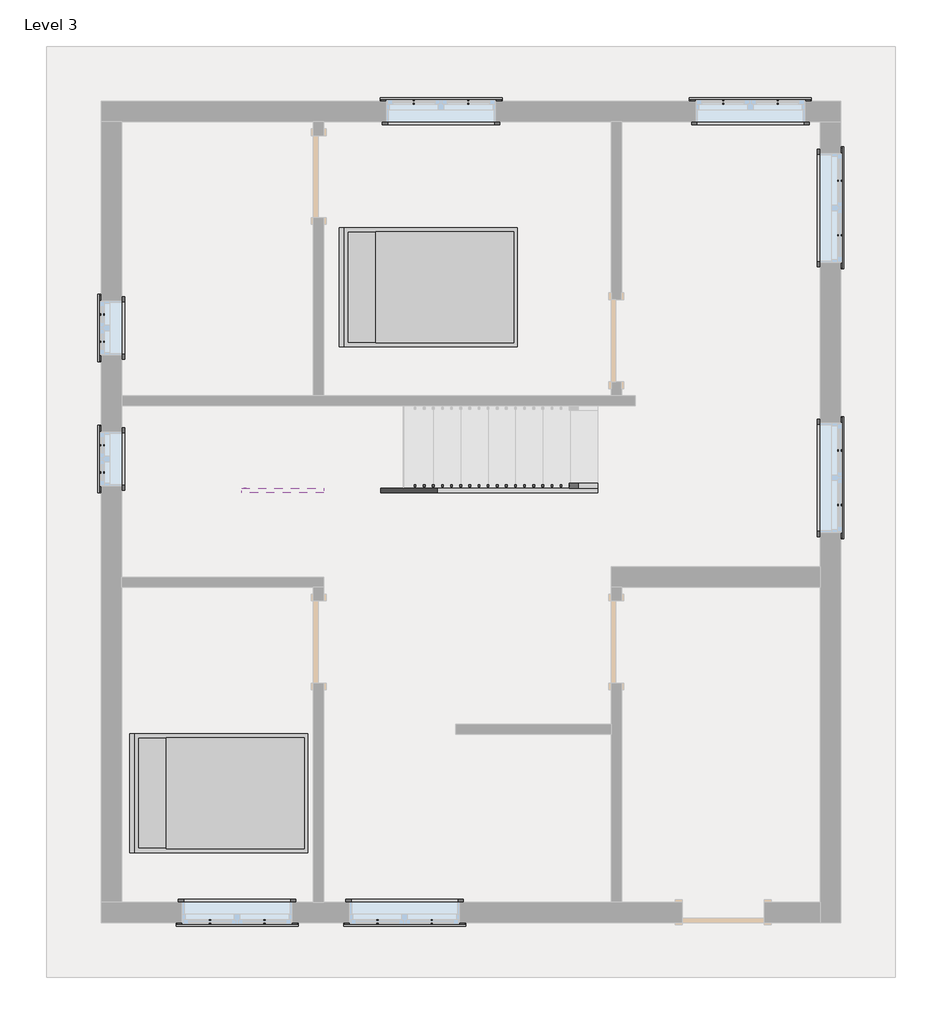
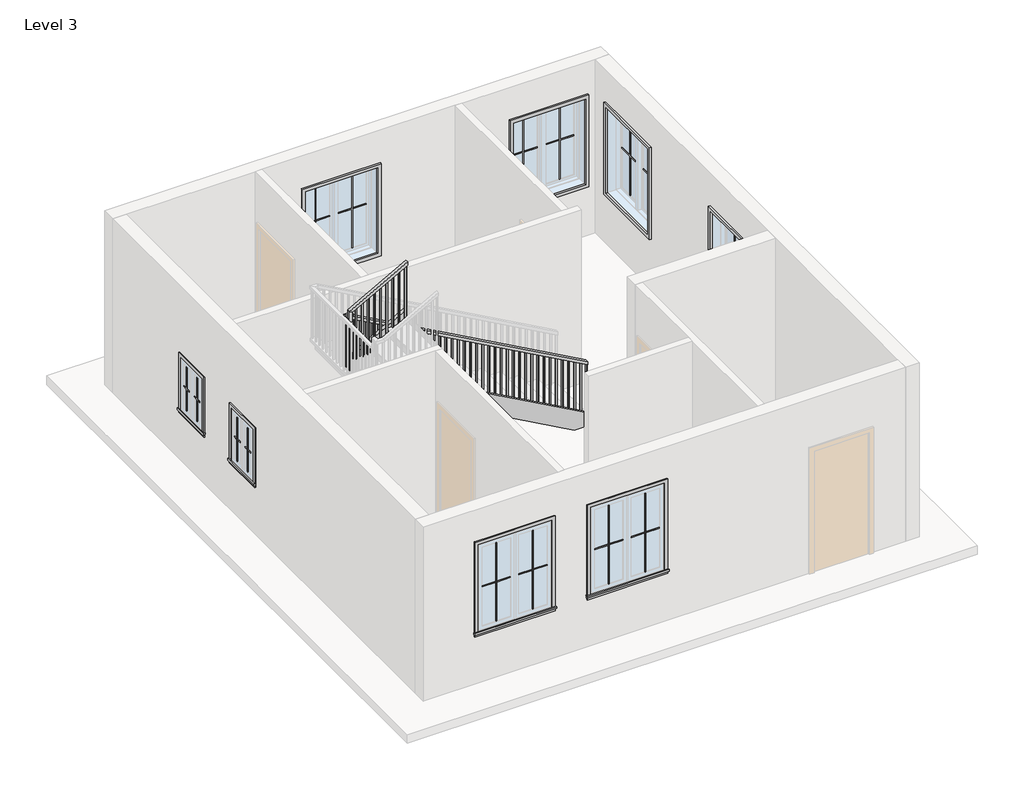
# One storey, part 2 of 2: 32 proxies, 3 members, 2 furniture elements, 1 railing.
"""IFC4 building model written with IfcOpenShell, lengths in millimetres."""

from ifc_helpers import new_model, si_unit, frame, origin, place, context, project, spatial, polyline, outline, extrude, faceted_brep, transform, mapped, element, save
from components import muntin_pattern_2x2_muntin_pattern_2x2_53152e2c, muntin_pattern_2x2_muntin_pattern_2x2_e8f3e573, muntin_pattern_2x2_muntin_pattern_2x2_6dad3731, muntin_pattern_2x2_muntin_pattern_2x2_a30a3345, trim_window_exterior_flat_with_sill_a665a915, trim_window_exterior_flat_with_sill_92b9b949, trim_window_interior_flat_picture_frame_d485c387, trim_window_interior_flat_picture_frame_3bb882cf, bed_17739_bed_17739_15c61121

model = new_model("IFC4")

# Units and contexts
model_context = context("Model", 3, world=origin())
ifc_project = project(units=[si_unit("LENGTHUNIT", "METRE", prefix="MILLI")], contexts=[model_context])

# Site, building, storey
site = spatial("IfcSite", under=ifc_project)
building = spatial("IfcBuilding", under=site)
storey = spatial("IfcBuildingStorey", under=building, Name="Level 3", Elevation=6096.0)

# Proxies
placement = place(None, origin())
muntin_pattern_2x2_muntin_pattern_2x2_shape = muntin_pattern_2x2_muntin_pattern_2x2_53152e2c(model_context)
element("IfcBuildingElementProxy", 1, Name="Muntin Pattern_2x2 : Muntin Pattern_2x2", ObjectType="Muntin Pattern_2x2 : Muntin Pattern_2x2", at=placement, inside=storey, context=model_context, shape_type="MappedRepresentation", body=[
    mapped(muntin_pattern_2x2_muntin_pattern_2x2_shape, transform((1279.525, 12101.9997886, 7080.25), x_axis=(0.0, 1.0, 0.0), y_axis=(-1.0, 0.0, 0.0), z_axis=(0.0, 0.0, 1.0))),
])
element("IfcBuildingElementProxy", 2, Name="Muntin Pattern_2x2 : Muntin Pattern_2x2", ObjectType="Muntin Pattern_2x2 : Muntin Pattern_2x2", at=placement, inside=storey, context=model_context, shape_type="MappedRepresentation", body=[
    mapped(muntin_pattern_2x2_muntin_pattern_2x2_shape, transform((1279.525, 10644.6747886, 7080.25), x_axis=(0.0, 1.0, 0.0), y_axis=(-1.0, 0.0, 0.0), z_axis=(0.0, 0.0, 1.0))),
])
muntin_pattern_2x2_muntin_pattern_2x2_2_shape = muntin_pattern_2x2_muntin_pattern_2x2_e8f3e573(model_context)
element("IfcBuildingElementProxy", 3, Name="Muntin Pattern_2x2 : Muntin Pattern_2x2", ObjectType="Muntin Pattern_2x2 : Muntin Pattern_2x2", at=placement, inside=storey, context=model_context, shape_type="MappedRepresentation", body=[
    mapped(muntin_pattern_2x2_muntin_pattern_2x2_2_shape, transform((1279.525, 12403.6247886, 7080.25), x_axis=(0.0, -1.0, 0.0), y_axis=(1.0, 0.0, 0.0), z_axis=(0.0, 0.0, 1.0))),
])
element("IfcBuildingElementProxy", 4, Name="Muntin Pattern_2x2 : Muntin Pattern_2x2", ObjectType="Muntin Pattern_2x2 : Muntin Pattern_2x2", at=placement, inside=storey, context=model_context, shape_type="MappedRepresentation", body=[
    mapped(muntin_pattern_2x2_muntin_pattern_2x2_2_shape, transform((1279.525, 10946.2997886, 7080.25), x_axis=(0.0, -1.0, 0.0), y_axis=(1.0, 0.0, 0.0), z_axis=(0.0, 0.0, 1.0))),
])
muntin_pattern_2x2_muntin_pattern_2x2_3_shape = muntin_pattern_2x2_muntin_pattern_2x2_6dad3731(model_context)
element("IfcBuildingElementProxy", 5, Name="Muntin Pattern_2x2 : Muntin Pattern_2x2", ObjectType="Muntin Pattern_2x2 : Muntin Pattern_2x2", at=placement, inside=storey, context=model_context, shape_type="MappedRepresentation", body=[
    mapped(muntin_pattern_2x2_muntin_pattern_2x2_3_shape, transform((9490.075, 13892.6997886, 7080.25), x_axis=(0.0, -1.0, 0.0), y_axis=(1.0, 0.0, 0.0), z_axis=(0.0, 0.0, 1.0))),
])
element("IfcBuildingElementProxy", 6, Name="Muntin Pattern_2x2 : Muntin Pattern_2x2", ObjectType="Muntin Pattern_2x2 : Muntin Pattern_2x2", at=placement, inside=storey, context=model_context, shape_type="MappedRepresentation", body=[
    mapped(muntin_pattern_2x2_muntin_pattern_2x2_3_shape, transform((8193.0875, 14767.4122886, 7080.25), x_axis=(1.0, 0.0, 0.0), y_axis=(0.0, 1.0, 0.0), z_axis=(0.0, 0.0, 1.0))),
])
element("IfcBuildingElementProxy", 7, Name="Muntin Pattern_2x2 : Muntin Pattern_2x2", ObjectType="Muntin Pattern_2x2 : Muntin Pattern_2x2", at=placement, inside=storey, context=model_context, shape_type="MappedRepresentation", body=[
    mapped(muntin_pattern_2x2_muntin_pattern_2x2_3_shape, transform((4749.8, 14767.4122886, 7080.25), x_axis=(1.0, 0.0, 0.0), y_axis=(0.0, 1.0, 0.0), z_axis=(0.0, 0.0, 1.0))),
])
element("IfcBuildingElementProxy", 8, Name="Muntin Pattern_2x2 : Muntin Pattern_2x2", ObjectType="Muntin Pattern_2x2 : Muntin Pattern_2x2", at=placement, inside=storey, context=model_context, shape_type="MappedRepresentation", body=[
    mapped(muntin_pattern_2x2_muntin_pattern_2x2_3_shape, transform((9490.075, 10889.1497886, 7080.25), x_axis=(0.0, -1.0, 0.0), y_axis=(1.0, 0.0, 0.0), z_axis=(0.0, 0.0, 1.0))),
])
element("IfcBuildingElementProxy", 9, Name="Muntin Pattern_2x2 : Muntin Pattern_2x2", ObjectType="Muntin Pattern_2x2 : Muntin Pattern_2x2", at=placement, inside=storey, context=model_context, shape_type="MappedRepresentation", body=[
    mapped(muntin_pattern_2x2_muntin_pattern_2x2_3_shape, transform((4950.6207347, 5642.4622886, 7080.25), x_axis=(-1.0, 0.0, 0.0), y_axis=(0.0, -1.0, 0.0), z_axis=(0.0, 0.0, 1.0))),
])
element("IfcBuildingElementProxy", 10, Name="Muntin Pattern_2x2 : Muntin Pattern_2x2", ObjectType="Muntin Pattern_2x2 : Muntin Pattern_2x2", at=placement, inside=storey, context=model_context, shape_type="MappedRepresentation", body=[
    mapped(muntin_pattern_2x2_muntin_pattern_2x2_3_shape, transform((3086.1019847, 5642.4622886, 7080.25), x_axis=(-1.0, 0.0, 0.0), y_axis=(0.0, -1.0, 0.0), z_axis=(0.0, 0.0, 1.0))),
])
muntin_pattern_2x2_muntin_pattern_2x2_4_shape = muntin_pattern_2x2_muntin_pattern_2x2_a30a3345(model_context)
element("IfcBuildingElementProxy", 11, Name="Muntin Pattern_2x2 : Muntin Pattern_2x2", ObjectType="Muntin Pattern_2x2 : Muntin Pattern_2x2", at=placement, inside=storey, context=model_context, shape_type="MappedRepresentation", body=[
    mapped(muntin_pattern_2x2_muntin_pattern_2x2_4_shape, transform((9490.075, 13286.2747886, 7080.25), x_axis=(0.0, 1.0, 0.0), y_axis=(-1.0, 0.0, 0.0), z_axis=(0.0, 0.0, 1.0))),
])
element("IfcBuildingElementProxy", 12, Name="Muntin Pattern_2x2 : Muntin Pattern_2x2", ObjectType="Muntin Pattern_2x2 : Muntin Pattern_2x2", at=placement, inside=storey, context=model_context, shape_type="MappedRepresentation", body=[
    mapped(muntin_pattern_2x2_muntin_pattern_2x2_4_shape, transform((8799.5125, 14767.4122886, 7080.25), x_axis=(-1.0, 0.0, 0.0), y_axis=(0.0, -1.0, 0.0), z_axis=(0.0, 0.0, 1.0))),
])
element("IfcBuildingElementProxy", 13, Name="Muntin Pattern_2x2 : Muntin Pattern_2x2", ObjectType="Muntin Pattern_2x2 : Muntin Pattern_2x2", at=placement, inside=storey, context=model_context, shape_type="MappedRepresentation", body=[
    mapped(muntin_pattern_2x2_muntin_pattern_2x2_4_shape, transform((5356.225, 14767.4122886, 7080.25), x_axis=(-1.0, 0.0, 0.0), y_axis=(0.0, -1.0, 0.0), z_axis=(0.0, 0.0, 1.0))),
])
element("IfcBuildingElementProxy", 14, Name="Muntin Pattern_2x2 : Muntin Pattern_2x2", ObjectType="Muntin Pattern_2x2 : Muntin Pattern_2x2", at=placement, inside=storey, context=model_context, shape_type="MappedRepresentation", body=[
    mapped(muntin_pattern_2x2_muntin_pattern_2x2_4_shape, transform((9490.075, 10282.7247886, 7080.25), x_axis=(0.0, 1.0, 0.0), y_axis=(-1.0, 0.0, 0.0), z_axis=(0.0, 0.0, 1.0))),
])
element("IfcBuildingElementProxy", 15, Name="Muntin Pattern_2x2 : Muntin Pattern_2x2", ObjectType="Muntin Pattern_2x2 : Muntin Pattern_2x2", at=placement, inside=storey, context=model_context, shape_type="MappedRepresentation", body=[
    mapped(muntin_pattern_2x2_muntin_pattern_2x2_4_shape, transform((4344.1957347, 5642.4622886, 7080.25), x_axis=(1.0, 0.0, 0.0), y_axis=(0.0, 1.0, 0.0), z_axis=(0.0, 0.0, 1.0))),
])
element("IfcBuildingElementProxy", 16, Name="Muntin Pattern_2x2 : Muntin Pattern_2x2", ObjectType="Muntin Pattern_2x2 : Muntin Pattern_2x2", at=placement, inside=storey, context=model_context, shape_type="MappedRepresentation", body=[
    mapped(muntin_pattern_2x2_muntin_pattern_2x2_4_shape, transform((2479.6769847, 5642.4622886, 7080.25), x_axis=(1.0, 0.0, 0.0), y_axis=(0.0, 1.0, 0.0), z_axis=(0.0, 0.0, 1.0))),
])
trim_window_exterior_flat_with_sill_shape = trim_window_exterior_flat_with_sill_a665a915(model_context)
element("IfcBuildingElementProxy", 17, Name="Trim-Window-Exterior-Flat : with Sill", ObjectType="Trim-Window-Exterior-Flat : with Sill", at=placement, inside=storey, context=model_context, shape_type="MappedRepresentation", body=[
    mapped(trim_window_exterior_flat_with_sill_shape, transform((1270.0, 12252.8122886, 7924.8), x_axis=(0.0, -1.0, 0.0), y_axis=(0.0, 0.0, 1.0), z_axis=(-1.0, 0.0, 0.0))),
])
element("IfcBuildingElementProxy", 18, Name="Trim-Window-Exterior-Flat : with Sill", ObjectType="Trim-Window-Exterior-Flat : with Sill", at=placement, inside=storey, context=model_context, shape_type="MappedRepresentation", body=[
    mapped(trim_window_exterior_flat_with_sill_shape, transform((1270.0, 10795.4872886, 7924.8), x_axis=(0.0, -1.0, 0.0), y_axis=(0.0, 0.0, 1.0), z_axis=(-1.0, 0.0, 0.0))),
])
trim_window_exterior_flat_with_sill_2_shape = trim_window_exterior_flat_with_sill_92b9b949(model_context)
element("IfcBuildingElementProxy", 19, Name="Trim-Window-Exterior-Flat : with Sill", ObjectType="Trim-Window-Exterior-Flat : with Sill", at=placement, inside=storey, context=model_context, shape_type="MappedRepresentation", body=[
    mapped(trim_window_exterior_flat_with_sill_2_shape, transform((9499.6, 13589.4872886, 8534.4), x_axis=(0.0, 1.0, 0.0), y_axis=(0.0, 0.0, 1.0), z_axis=(1.0, 0.0, 0.0))),
])
element("IfcBuildingElementProxy", 20, Name="Trim-Window-Exterior-Flat : with Sill", ObjectType="Trim-Window-Exterior-Flat : with Sill", at=placement, inside=storey, context=model_context, shape_type="MappedRepresentation", body=[
    mapped(trim_window_exterior_flat_with_sill_2_shape, transform((8496.3, 14776.9372886, 8534.4), x_axis=(-1.0, 0.0, 0.0), y_axis=(0.0, 0.0, 1.0), z_axis=(0.0, 1.0, 0.0))),
])
element("IfcBuildingElementProxy", 21, Name="Trim-Window-Exterior-Flat : with Sill", ObjectType="Trim-Window-Exterior-Flat : with Sill", at=placement, inside=storey, context=model_context, shape_type="MappedRepresentation", body=[
    mapped(trim_window_exterior_flat_with_sill_2_shape, transform((5053.0125, 14776.9372886, 8534.4), x_axis=(-1.0, 0.0, 0.0), y_axis=(0.0, 0.0, 1.0), z_axis=(0.0, 1.0, 0.0))),
])
element("IfcBuildingElementProxy", 22, Name="Trim-Window-Exterior-Flat : with Sill", ObjectType="Trim-Window-Exterior-Flat : with Sill", at=placement, inside=storey, context=model_context, shape_type="MappedRepresentation", body=[
    mapped(trim_window_exterior_flat_with_sill_2_shape, transform((9499.6, 10585.9372886, 8534.4), x_axis=(0.0, 1.0, 0.0), y_axis=(0.0, 0.0, 1.0), z_axis=(1.0, 0.0, 0.0))),
])
element("IfcBuildingElementProxy", 23, Name="Trim-Window-Exterior-Flat : with Sill", ObjectType="Trim-Window-Exterior-Flat : with Sill", at=placement, inside=storey, context=model_context, shape_type="MappedRepresentation", body=[
    mapped(trim_window_exterior_flat_with_sill_2_shape, transform((4647.4082347, 5632.9372886, 8534.4), x_axis=(1.0, 0.0, 0.0), y_axis=(0.0, 0.0, 1.0), z_axis=(0.0, -1.0, 0.0))),
])
element("IfcBuildingElementProxy", 24, Name="Trim-Window-Exterior-Flat : with Sill", ObjectType="Trim-Window-Exterior-Flat : with Sill", at=placement, inside=storey, context=model_context, shape_type="MappedRepresentation", body=[
    mapped(trim_window_exterior_flat_with_sill_2_shape, transform((2782.8894847, 5632.9372886, 8534.4), x_axis=(1.0, 0.0, 0.0), y_axis=(0.0, 0.0, 1.0), z_axis=(0.0, -1.0, 0.0))),
])
trim_window_interior_flat_picture_frame_shape = trim_window_interior_flat_picture_frame_d485c387(model_context)
element("IfcBuildingElementProxy", 25, Name="Trim-Window-Interior-Flat : Picture Frame", ObjectType="Trim-Window-Interior-Flat : Picture Frame", at=placement, inside=storey, context=model_context, shape_type="MappedRepresentation", body=[
    mapped(trim_window_interior_flat_picture_frame_shape, transform((1498.6, 12252.8122886, 7924.8), x_axis=(0.0, 1.0, 0.0), y_axis=(0.0, 0.0, 1.0), z_axis=(1.0, 0.0, 0.0))),
])
element("IfcBuildingElementProxy", 26, Name="Trim-Window-Interior-Flat : Picture Frame", ObjectType="Trim-Window-Interior-Flat : Picture Frame", at=placement, inside=storey, context=model_context, shape_type="MappedRepresentation", body=[
    mapped(trim_window_interior_flat_picture_frame_shape, transform((1498.6, 10795.4872886, 7924.8), x_axis=(0.0, 1.0, 0.0), y_axis=(0.0, 0.0, 1.0), z_axis=(1.0, 0.0, 0.0))),
])
trim_window_interior_flat_picture_frame_2_shape = trim_window_interior_flat_picture_frame_3bb882cf(model_context)
element("IfcBuildingElementProxy", 27, Name="Trim-Window-Interior-Flat : Picture Frame", ObjectType="Trim-Window-Interior-Flat : Picture Frame", at=placement, inside=storey, context=model_context, shape_type="MappedRepresentation", body=[
    mapped(trim_window_interior_flat_picture_frame_2_shape, transform((9271.0, 13589.4872886, 8534.4), x_axis=(0.0, -1.0, 0.0), y_axis=(0.0, 0.0, 1.0), z_axis=(-1.0, 0.0, 0.0))),
])
element("IfcBuildingElementProxy", 28, Name="Trim-Window-Interior-Flat : Picture Frame", ObjectType="Trim-Window-Interior-Flat : Picture Frame", at=placement, inside=storey, context=model_context, shape_type="MappedRepresentation", body=[
    mapped(trim_window_interior_flat_picture_frame_2_shape, transform((8496.3, 14548.3372886, 8534.4), x_axis=(1.0, 0.0, 0.0), y_axis=(0.0, 0.0, 1.0), z_axis=(0.0, -1.0, 0.0))),
])
element("IfcBuildingElementProxy", 29, Name="Trim-Window-Interior-Flat : Picture Frame", ObjectType="Trim-Window-Interior-Flat : Picture Frame", at=placement, inside=storey, context=model_context, shape_type="MappedRepresentation", body=[
    mapped(trim_window_interior_flat_picture_frame_2_shape, transform((5053.0125, 14548.3372886, 8534.4), x_axis=(1.0, 0.0, 0.0), y_axis=(0.0, 0.0, 1.0), z_axis=(0.0, -1.0, 0.0))),
])
element("IfcBuildingElementProxy", 30, Name="Trim-Window-Interior-Flat : Picture Frame", ObjectType="Trim-Window-Interior-Flat : Picture Frame", at=placement, inside=storey, context=model_context, shape_type="MappedRepresentation", body=[
    mapped(trim_window_interior_flat_picture_frame_2_shape, transform((9271.0, 10585.9372886, 8534.4), x_axis=(0.0, -1.0, 0.0), y_axis=(0.0, 0.0, 1.0), z_axis=(-1.0, 0.0, 0.0))),
])
element("IfcBuildingElementProxy", 31, Name="Trim-Window-Interior-Flat : Picture Frame", ObjectType="Trim-Window-Interior-Flat : Picture Frame", at=placement, inside=storey, context=model_context, shape_type="MappedRepresentation", body=[
    mapped(trim_window_interior_flat_picture_frame_2_shape, transform((4647.4082347, 5861.5372886, 8534.4), x_axis=(-1.0, 0.0, 0.0), y_axis=(0.0, 0.0, 1.0), z_axis=(0.0, 1.0, 0.0))),
])
element("IfcBuildingElementProxy", 32, Name="Trim-Window-Interior-Flat : Picture Frame", ObjectType="Trim-Window-Interior-Flat : Picture Frame", at=placement, inside=storey, context=model_context, shape_type="MappedRepresentation", body=[
    mapped(trim_window_interior_flat_picture_frame_2_shape, transform((2782.8894847, 5861.5372886, 8534.4), x_axis=(-1.0, 0.0, 0.0), y_axis=(0.0, 0.0, 1.0), z_axis=(0.0, 1.0, 0.0))),
])

# Furniture
bed_17739_bed_17739_shape = bed_17739_bed_17739_15c61121(model_context)
element("IfcFurniture", 33, ObjectType="Bed_17739 : Bed_17739", at=placement, inside=storey, context=model_context, shape_type="MappedRepresentation", body=[
    mapped(bed_17739_bed_17739_shape, transform((4933.95, 12706.8372886, 6096.0), x_axis=(0.0, 1.0, 0.0), y_axis=(-1.0, 0.0, 0.0), z_axis=(0.0, 0.0, 1.0))),
])
element("IfcFurniture", 34, ObjectType="Bed_17739 : Bed_17739", at=placement, inside=storey, context=model_context, shape_type="MappedRepresentation", body=[
    mapped(bed_17739_bed_17739_shape, transform((2603.5, 7074.3872886, 6096.0), x_axis=(0.0, 1.0, 0.0), y_axis=(-1.0, 0.0, 0.0), z_axis=(0.0, 0.0, 1.0))),
])

# Members
element("IfcMember", 35, ObjectType="Stringer - 2\" Width", at=placement, inside=storey, context=model_context, shape_type="SweptSolid", body=[
    extrude(outline(polyline([(6096.0, 6794.5), (6303.5983948, 6794.5), (8476.7095059, 2882.9), (8128.0308318, 2882.9), (6096.0, 6540.5554972), (6096.0, 6794.5)])), frame((0.0, 10420.8372886, 0.0), z_axis=(0.0, 1.0, 0.0), x_axis=(0.0, 0.0, 1.0)), (0.0, 0.0, 1.0), 50.8),
])
element("IfcMember", 36, ObjectType="Stringer - 2\" Width", at=placement, inside=storey, context=model_context, shape_type="SweptSolid", body=[
    extrude(outline(polyline([(2832.1, 10471.6372886), (2882.9, 10471.6372886), (2882.9, 10469.0972886), (2832.1, 10469.0972886), (2832.1, 10471.6372886)])), frame((0.0, 0.0, 8238.0666667), z_axis=(0.0, 0.0, 1.0), x_axis=(1.0, 0.0, 0.0)), (0.0, 0.0, 1.0), 304.8),
])
element("IfcMember", 37, ObjectType="Stringer - 2\" Width", at=placement, inside=storey, context=model_context, shape_type="SweptSolid", body=[
    extrude(outline(polyline([(8674.2650614, 2832.1), (8325.5863873, 2832.1), (8833.5874899, 3746.5019847), (9182.266164, 3746.5019847), (8674.2650614, 2832.1)])), frame((0.0, 10418.2972886, 0.0), z_axis=(0.0, 1.0, 0.0), x_axis=(0.0, 0.0, 1.0)), (0.0, 0.0, 1.0), 50.8),
])

# Railing
element("IfcRailing", 38, ObjectType="Handrail - Rectangular", at=placement, inside=storey, context=model_context, shape_type="SolidModel", body=[
    faceted_brep([(6794.5, 10471.6372886, 7179.7333333), (6794.5, 10471.6372886, 7121.620221), (6794.5, 10522.4372886, 7121.620221), (6794.5, 10522.4372886, 7179.7333333), (2908.3, 10471.6372886, 9338.7333333), (2857.5, 10471.6372886, 9308.8424432), (2857.5, 10522.4372886, 9308.8424432), (2908.3, 10522.4372886, 9338.7333333), (2908.3, 10471.6372886, 9381.0666667), (2857.5, 10471.6372886, 9330.2666667), (2857.5, 10522.4372886, 9330.2666667), (2908.3, 10522.4372886, 9381.0666667), (2832.1, 10471.6372886, 9381.0666667), (2832.1, 10471.6372886, 9330.2666667), (2781.3, 10522.4372886, 9330.2666667), (2781.3, 10522.4372886, 9381.0666667), (2832.1, 10395.4372886, 9381.0666667), (2832.1, 10395.4372886, 9330.2666667), (2781.3, 10395.4372886, 9330.2666667), (2781.3, 10395.4372886, 9381.0666667), (2832.1, 10392.8972886, 9381.0666667), (2781.3, 10392.8972886, 9381.0666667), (2781.3, 10392.8972886, 9330.2666667), (2832.1, 10392.8972886, 9330.2666667)], [[[0, 1, 2, 3]], [[1, 0, 4, 5]], [[2, 1, 5, 6]], [[3, 2, 6, 7]], [[0, 3, 7, 4]], [[5, 4, 8, 9]], [[6, 5, 9, 10]], [[7, 6, 10, 11]], [[4, 7, 11, 8]], [[9, 8, 12, 13]], [[10, 9, 13, 14]], [[11, 10, 14, 15]], [[8, 11, 15, 12]], [[13, 12, 16, 17]], [[14, 13, 17, 18]], [[15, 14, 18, 19]], [[12, 15, 19, 16]], [[20, 21, 22, 23]], [[17, 16, 20, 23]], [[18, 17, 23, 22]], [[19, 18, 22, 21]], [[16, 19, 21, 20]]]),
    faceted_brep([(2832.1, 10418.2972886, 9381.0666667), (2832.1, 10367.4972886, 9330.2666667), (2781.3, 10367.4972886, 9330.2666667), (2781.3, 10418.2972886, 9381.0666667), (2832.1, 10418.2972886, 9492.2869174), (2781.3, 10418.2972886, 9522.177839), (2781.3, 10367.4972886, 9522.177839), (2832.1, 10367.4972886, 9492.2869174)], [[[0, 1, 2, 3]], [[4, 5, 6, 7]], [[1, 0, 4, 7]], [[2, 1, 7, 6]], [[3, 2, 6, 5]], [[0, 3, 5, 4]]]),
    faceted_brep([(2781.3, 10418.2972886, 9522.177839), (2832.1, 10418.2972886, 9492.2869174), (2832.1, 10367.4972886, 9492.2869174), (2781.3, 10367.4972886, 9522.177839), (3746.5019847, 10418.2972886, 10058.4), (3746.5019847, 10367.4972886, 10058.4), (3746.5019847, 10367.4972886, 10000.2869174), (3746.5019847, 10418.2972886, 10000.2869174)], [[[0, 1, 2, 3]], [[4, 5, 6, 7]], [[1, 0, 4, 7]], [[2, 1, 7, 6]], [[3, 2, 6, 5]], [[0, 3, 5, 4]]]),
    extrude(outline(polyline([(9980.8838142, 3711.575), (8974.6666667, 3711.575), (8974.6666667, 3730.625), (9991.4671246, 3730.625), (9980.8838142, 3711.575)])), frame((0.0, 10383.3722886, 0.0), z_axis=(0.0, 1.0, 0.0), x_axis=(0.0, 0.0, 1.0)), (0.0, 0.0, 1.0), 19.05),
    extrude(outline(polyline([(9924.4394923, 3609.975), (8974.6666667, 3609.975), (8974.6666667, 3629.025), (9935.0228026, 3629.025), (9924.4394923, 3609.975)])), frame((0.0, 10383.3722886, 0.0), z_axis=(0.0, 1.0, 0.0), x_axis=(0.0, 0.0, 1.0)), (0.0, 0.0, 1.0), 19.05),
    extrude(outline(polyline([(9867.9951703, 3508.375), (8974.6666667, 3508.375), (8974.6666667, 3527.425), (9878.5784807, 3527.425), (9867.9951703, 3508.375)])), frame((0.0, 10383.3722886, 0.0), z_axis=(0.0, 1.0, 0.0), x_axis=(0.0, 0.0, 1.0)), (0.0, 0.0, 1.0), 19.05),
    extrude(outline(polyline([(9811.5504809, 3406.775), (8805.3333333, 3406.775), (8805.3333333, 3425.825), (9822.1337912, 3425.825), (9811.5504809, 3406.775)])), frame((0.0, 10383.3722886, 0.0), z_axis=(0.0, 1.0, 0.0), x_axis=(0.0, 0.0, 1.0)), (0.0, 0.0, 1.0), 19.05),
    extrude(outline(polyline([(9755.1061589, 3305.175), (8805.3333333, 3305.175), (8805.3333333, 3324.225), (9765.6894693, 3324.225), (9755.1061589, 3305.175)])), frame((0.0, 10383.3722886, 0.0), z_axis=(0.0, 1.0, 0.0), x_axis=(0.0, 0.0, 1.0)), (0.0, 0.0, 1.0), 19.05),
    extrude(outline(polyline([(9698.661837, 3203.575), (8805.3333333, 3203.575), (8805.3333333, 3222.625), (9709.2451474, 3222.625), (9698.661837, 3203.575)])), frame((0.0, 10383.3722886, 0.0), z_axis=(0.0, 1.0, 0.0), x_axis=(0.0, 0.0, 1.0)), (0.0, 0.0, 1.0), 19.05),
    extrude(outline(polyline([(9642.2171475, 3101.975), (8636.0, 3101.975), (8636.0, 3121.025), (9652.8004579, 3121.025), (9642.2171475, 3101.975)])), frame((0.0, 10383.3722886, 0.0), z_axis=(0.0, 1.0, 0.0), x_axis=(0.0, 0.0, 1.0)), (0.0, 0.0, 1.0), 19.05),
    extrude(outline(polyline([(9585.7728256, 3000.375), (8636.0, 3000.375), (8636.0, 3019.425), (9596.356136, 3019.425), (9585.7728256, 3000.375)])), frame((0.0, 10383.3722886, 0.0), z_axis=(0.0, 1.0, 0.0), x_axis=(0.0, 0.0, 1.0)), (0.0, 0.0, 1.0), 19.05),
    extrude(outline(polyline([(9529.3285037, 2898.775), (8636.0, 2898.775), (8636.0, 2917.825), (9539.911814, 2917.825), (9529.3285037, 2898.775)])), frame((0.0, 10383.3722886, 0.0), z_axis=(0.0, 1.0, 0.0), x_axis=(0.0, 0.0, 1.0)), (0.0, 0.0, 1.0), 19.05),
    extrude(outline(polyline([(2816.225, 10404.9622886), (2816.225, 10385.9122886), (2797.175, 10385.9122886), (2797.175, 10404.9622886), (2816.225, 10404.9622886)])), frame((0.0, 0.0, 8466.6666667), z_axis=(0.0, 0.0, 1.0), x_axis=(1.0, 0.0, 0.0)), (0.0, 0.0, 1.0), 863.6),
    extrude(outline(polyline([(2841.625, 10487.5122886), (2822.575, 10487.5122886), (2822.575, 10506.5622886), (2841.625, 10506.5622886), (2841.625, 10487.5122886)])), frame((0.0, 0.0, 8466.6666667), z_axis=(0.0, 0.0, 1.0), x_axis=(1.0, 0.0, 0.0)), (0.0, 0.0, 1.0), 863.6),
    extrude(outline(polyline([(9271.8007765, 2924.175), (8297.3333333, 2924.175), (8297.3333333, 2943.225), (9261.2174432, 2943.225), (9271.8007765, 2924.175)])), frame((0.0, 10487.5122886, 0.0), z_axis=(0.0, 1.0, 0.0), x_axis=(0.0, 0.0, 1.0)), (0.0, 0.0, 1.0), 19.05),
    extrude(outline(polyline([(9215.3563321, 3025.775), (8297.3333333, 3025.775), (8297.3333333, 3044.825), (9204.7729988, 3044.825), (9215.3563321, 3025.775)])), frame((0.0, 10487.5122886, 0.0), z_axis=(0.0, 1.0, 0.0), x_axis=(0.0, 0.0, 1.0)), (0.0, 0.0, 1.0), 19.05),
    extrude(outline(polyline([(9158.9118876, 3127.375), (8297.3333333, 3127.375), (8297.3333333, 3146.425), (9148.3285543, 3146.425), (9158.9118876, 3127.375)])), frame((0.0, 10487.5122886, 0.0), z_axis=(0.0, 1.0, 0.0), x_axis=(0.0, 0.0, 1.0)), (0.0, 0.0, 1.0), 19.05),
    extrude(outline(polyline([(9102.4674432, 3228.975), (8128.0, 3228.975), (8128.0, 3248.025), (9091.8841099, 3248.025), (9102.4674432, 3228.975)])), frame((0.0, 10487.5122886, 0.0), z_axis=(0.0, 1.0, 0.0), x_axis=(0.0, 0.0, 1.0)), (0.0, 0.0, 1.0), 19.05),
    extrude(outline(polyline([(9046.0229988, 3330.575), (8128.0, 3330.575), (8128.0, 3349.625), (9035.4396654, 3349.625), (9046.0229988, 3330.575)])), frame((0.0, 10487.5122886, 0.0), z_axis=(0.0, 1.0, 0.0), x_axis=(0.0, 0.0, 1.0)), (0.0, 0.0, 1.0), 19.05),
    extrude(outline(polyline([(8989.5785543, 3432.175), (8128.0, 3432.175), (8128.0, 3451.225), (8978.995221, 3451.225), (8989.5785543, 3432.175)])), frame((0.0, 10487.5122886, 0.0), z_axis=(0.0, 1.0, 0.0), x_axis=(0.0, 0.0, 1.0)), (0.0, 0.0, 1.0), 19.05),
    extrude(outline(polyline([(8933.1341099, 3533.775), (7958.6666667, 3533.775), (7958.6666667, 3552.825), (8922.5507765, 3552.825), (8933.1341099, 3533.775)])), frame((0.0, 10487.5122886, 0.0), z_axis=(0.0, 1.0, 0.0), x_axis=(0.0, 0.0, 1.0)), (0.0, 0.0, 1.0), 19.05),
    extrude(outline(polyline([(8876.6896654, 3635.375), (7958.6666667, 3635.375), (7958.6666667, 3654.425), (8866.1063321, 3654.425), (8876.6896654, 3635.375)])), frame((0.0, 10487.5122886, 0.0), z_axis=(0.0, 1.0, 0.0), x_axis=(0.0, 0.0, 1.0)), (0.0, 0.0, 1.0), 19.05),
    extrude(outline(polyline([(8820.245221, 3736.975), (7958.6666667, 3736.975), (7958.6666667, 3756.025), (8809.6618876, 3756.025), (8820.245221, 3736.975)])), frame((0.0, 10487.5122886, 0.0), z_axis=(0.0, 1.0, 0.0), x_axis=(0.0, 0.0, 1.0)), (0.0, 0.0, 1.0), 19.05),
    extrude(outline(polyline([(8763.8007765, 3838.575), (7789.3333333, 3838.575), (7789.3333333, 3857.625), (8753.2174432, 3857.625), (8763.8007765, 3838.575)])), frame((0.0, 10487.5122886, 0.0), z_axis=(0.0, 1.0, 0.0), x_axis=(0.0, 0.0, 1.0)), (0.0, 0.0, 1.0), 19.05),
    extrude(outline(polyline([(8707.3563321, 3940.175), (7789.3333333, 3940.175), (7789.3333333, 3959.225), (8696.7729988, 3959.225), (8707.3563321, 3940.175)])), frame((0.0, 10487.5122886, 0.0), z_axis=(0.0, 1.0, 0.0), x_axis=(0.0, 0.0, 1.0)), (0.0, 0.0, 1.0), 19.05),
    extrude(outline(polyline([(8650.9118876, 4041.775), (7789.3333333, 4041.775), (7789.3333333, 4060.825), (8640.3285543, 4060.825), (8650.9118876, 4041.775)])), frame((0.0, 10487.5122886, 0.0), z_axis=(0.0, 1.0, 0.0), x_axis=(0.0, 0.0, 1.0)), (0.0, 0.0, 1.0), 19.05),
    extrude(outline(polyline([(8594.4674432, 4143.375), (7620.0, 4143.375), (7620.0, 4162.425), (8583.8841099, 4162.425), (8594.4674432, 4143.375)])), frame((0.0, 10487.5122886, 0.0), z_axis=(0.0, 1.0, 0.0), x_axis=(0.0, 0.0, 1.0)), (0.0, 0.0, 1.0), 19.05),
    extrude(outline(polyline([(8538.0229988, 4244.975), (7620.0, 4244.975), (7620.0, 4264.025), (8527.4396654, 4264.025), (8538.0229988, 4244.975)])), frame((0.0, 10487.5122886, 0.0), z_axis=(0.0, 1.0, 0.0), x_axis=(0.0, 0.0, 1.0)), (0.0, 0.0, 1.0), 19.05),
    extrude(outline(polyline([(8481.5785543, 4346.575), (7620.0, 4346.575), (7620.0, 4365.625), (8470.995221, 4365.625), (8481.5785543, 4346.575)])), frame((0.0, 10487.5122886, 0.0), z_axis=(0.0, 1.0, 0.0), x_axis=(0.0, 0.0, 1.0)), (0.0, 0.0, 1.0), 19.05),
    extrude(outline(polyline([(8425.1341099, 4448.175), (7450.6666667, 4448.175), (7450.6666667, 4467.225), (8414.5507765, 4467.225), (8425.1341099, 4448.175)])), frame((0.0, 10487.5122886, 0.0), z_axis=(0.0, 1.0, 0.0), x_axis=(0.0, 0.0, 1.0)), (0.0, 0.0, 1.0), 19.05),
    extrude(outline(polyline([(8368.6896654, 4549.775), (7450.6666667, 4549.775), (7450.6666667, 4568.825), (8358.1063321, 4568.825), (8368.6896654, 4549.775)])), frame((0.0, 10487.5122886, 0.0), z_axis=(0.0, 1.0, 0.0), x_axis=(0.0, 0.0, 1.0)), (0.0, 0.0, 1.0), 19.05),
    extrude(outline(polyline([(8312.245221, 4651.375), (7450.6666667, 4651.375), (7450.6666667, 4670.425), (8301.6618876, 4670.425), (8312.245221, 4651.375)])), frame((0.0, 10487.5122886, 0.0), z_axis=(0.0, 1.0, 0.0), x_axis=(0.0, 0.0, 1.0)), (0.0, 0.0, 1.0), 19.05),
    extrude(outline(polyline([(8255.8007765, 4752.975), (7281.3333333, 4752.975), (7281.3333333, 4772.025), (8245.2174432, 4772.025), (8255.8007765, 4752.975)])), frame((0.0, 10487.5122886, 0.0), z_axis=(0.0, 1.0, 0.0), x_axis=(0.0, 0.0, 1.0)), (0.0, 0.0, 1.0), 19.05),
    extrude(outline(polyline([(8199.3563321, 4854.575), (7281.3333333, 4854.575), (7281.3333333, 4873.625), (8188.7729988, 4873.625), (8199.3563321, 4854.575)])), frame((0.0, 10487.5122886, 0.0), z_axis=(0.0, 1.0, 0.0), x_axis=(0.0, 0.0, 1.0)), (0.0, 0.0, 1.0), 19.05),
    extrude(outline(polyline([(8142.9118876, 4956.175), (7281.3333333, 4956.175), (7281.3333333, 4975.225), (8132.3285543, 4975.225), (8142.9118876, 4956.175)])), frame((0.0, 10487.5122886, 0.0), z_axis=(0.0, 1.0, 0.0), x_axis=(0.0, 0.0, 1.0)), (0.0, 0.0, 1.0), 19.05),
    extrude(outline(polyline([(8086.4674432, 5057.775), (7112.0, 5057.775), (7112.0, 5076.825), (8075.8841099, 5076.825), (8086.4674432, 5057.775)])), frame((0.0, 10487.5122886, 0.0), z_axis=(0.0, 1.0, 0.0), x_axis=(0.0, 0.0, 1.0)), (0.0, 0.0, 1.0), 19.05),
    extrude(outline(polyline([(8030.0229988, 5159.375), (7112.0, 5159.375), (7112.0, 5178.425), (8019.4396654, 5178.425), (8030.0229988, 5159.375)])), frame((0.0, 10487.5122886, 0.0), z_axis=(0.0, 1.0, 0.0), x_axis=(0.0, 0.0, 1.0)), (0.0, 0.0, 1.0), 19.05),
    extrude(outline(polyline([(7973.5785543, 5260.975), (7112.0, 5260.975), (7112.0, 5280.025), (7962.995221, 5280.025), (7973.5785543, 5260.975)])), frame((0.0, 10487.5122886, 0.0), z_axis=(0.0, 1.0, 0.0), x_axis=(0.0, 0.0, 1.0)), (0.0, 0.0, 1.0), 19.05),
    extrude(outline(polyline([(7917.1341099, 5362.575), (6942.6666667, 5362.575), (6942.6666667, 5381.625), (7906.5507765, 5381.625), (7917.1341099, 5362.575)])), frame((0.0, 10487.5122886, 0.0), z_axis=(0.0, 1.0, 0.0), x_axis=(0.0, 0.0, 1.0)), (0.0, 0.0, 1.0), 19.05),
    extrude(outline(polyline([(7860.6896654, 5464.175), (6942.6666667, 5464.175), (6942.6666667, 5483.225), (7850.1063321, 5483.225), (7860.6896654, 5464.175)])), frame((0.0, 10487.5122886, 0.0), z_axis=(0.0, 1.0, 0.0), x_axis=(0.0, 0.0, 1.0)), (0.0, 0.0, 1.0), 19.05),
    extrude(outline(polyline([(7804.245221, 5565.775), (6942.6666667, 5565.775), (6942.6666667, 5584.825), (7793.6618876, 5584.825), (7804.245221, 5565.775)])), frame((0.0, 10487.5122886, 0.0), z_axis=(0.0, 1.0, 0.0), x_axis=(0.0, 0.0, 1.0)), (0.0, 0.0, 1.0), 19.05),
    extrude(outline(polyline([(7747.8007765, 5667.375), (6773.3333333, 5667.375), (6773.3333333, 5686.425), (7737.2174432, 5686.425), (7747.8007765, 5667.375)])), frame((0.0, 10487.5122886, 0.0), z_axis=(0.0, 1.0, 0.0), x_axis=(0.0, 0.0, 1.0)), (0.0, 0.0, 1.0), 19.05),
    extrude(outline(polyline([(7691.3563321, 5768.975), (6773.3333333, 5768.975), (6773.3333333, 5788.025), (7680.7729988, 5788.025), (7691.3563321, 5768.975)])), frame((0.0, 10487.5122886, 0.0), z_axis=(0.0, 1.0, 0.0), x_axis=(0.0, 0.0, 1.0)), (0.0, 0.0, 1.0), 19.05),
    extrude(outline(polyline([(7634.9118876, 5870.575), (6773.3333333, 5870.575), (6773.3333333, 5889.625), (7624.3285543, 5889.625), (7634.9118876, 5870.575)])), frame((0.0, 10487.5122886, 0.0), z_axis=(0.0, 1.0, 0.0), x_axis=(0.0, 0.0, 1.0)), (0.0, 0.0, 1.0), 19.05),
    extrude(outline(polyline([(7578.4674432, 5972.175), (6604.0, 5972.175), (6604.0, 5991.225), (7567.8841099, 5991.225), (7578.4674432, 5972.175)])), frame((0.0, 10487.5122886, 0.0), z_axis=(0.0, 1.0, 0.0), x_axis=(0.0, 0.0, 1.0)), (0.0, 0.0, 1.0), 19.05),
    extrude(outline(polyline([(7522.0229988, 6073.775), (6604.0, 6073.775), (6604.0, 6092.825), (7511.4396654, 6092.825), (7522.0229988, 6073.775)])), frame((0.0, 10487.5122886, 0.0), z_axis=(0.0, 1.0, 0.0), x_axis=(0.0, 0.0, 1.0)), (0.0, 0.0, 1.0), 19.05),
    extrude(outline(polyline([(7465.5785543, 6175.375), (6604.0, 6175.375), (6604.0, 6194.425), (7454.995221, 6194.425), (7465.5785543, 6175.375)])), frame((0.0, 10487.5122886, 0.0), z_axis=(0.0, 1.0, 0.0), x_axis=(0.0, 0.0, 1.0)), (0.0, 0.0, 1.0), 19.05),
    extrude(outline(polyline([(7409.1341099, 6276.975), (6434.6666667, 6276.975), (6434.6666667, 6296.025), (7398.5507765, 6296.025), (7409.1341099, 6276.975)])), frame((0.0, 10487.5122886, 0.0), z_axis=(0.0, 1.0, 0.0), x_axis=(0.0, 0.0, 1.0)), (0.0, 0.0, 1.0), 19.05),
    extrude(outline(polyline([(7352.6896654, 6378.575), (6434.6666667, 6378.575), (6434.6666667, 6397.625), (7342.1063321, 6397.625), (7352.6896654, 6378.575)])), frame((0.0, 10487.5122886, 0.0), z_axis=(0.0, 1.0, 0.0), x_axis=(0.0, 0.0, 1.0)), (0.0, 0.0, 1.0), 19.05),
    extrude(outline(polyline([(7296.245221, 6480.175), (6434.6666667, 6480.175), (6434.6666667, 6499.225), (7285.6618876, 6499.225), (7296.245221, 6480.175)])), frame((0.0, 10487.5122886, 0.0), z_axis=(0.0, 1.0, 0.0), x_axis=(0.0, 0.0, 1.0)), (0.0, 0.0, 1.0), 19.05),
    extrude(outline(polyline([(7239.8007765, 6581.775), (6265.3333333, 6581.775), (6265.3333333, 6600.825), (7229.2174432, 6600.825), (7239.8007765, 6581.775)])), frame((0.0, 10487.5122886, 0.0), z_axis=(0.0, 1.0, 0.0), x_axis=(0.0, 0.0, 1.0)), (0.0, 0.0, 1.0), 19.05),
    extrude(outline(polyline([(7183.3563321, 6683.375), (6265.3333333, 6683.375), (6265.3333333, 6702.425), (7172.7729988, 6702.425), (7183.3563321, 6683.375)])), frame((0.0, 10487.5122886, 0.0), z_axis=(0.0, 1.0, 0.0), x_axis=(0.0, 0.0, 1.0)), (0.0, 0.0, 1.0), 19.05),
    extrude(outline(polyline([(2816.225, 10402.4222886), (2816.225, 10383.3722886), (2797.175, 10383.3722886), (2797.175, 10402.4222886), (2816.225, 10402.4222886)])), frame((0.0, 0.0, 8466.6666667), z_axis=(0.0, 0.0, 1.0), x_axis=(1.0, 0.0, 0.0)), (0.0, 0.0, 1.0), 863.6),
    extrude(outline(polyline([(2816.225, 10487.5122886), (2797.175, 10487.5122886), (2797.175, 10506.5622886), (2816.225, 10506.5622886), (2816.225, 10487.5122886)])), frame((0.0, 0.0, 8466.6666667), z_axis=(0.0, 0.0, 1.0), x_axis=(1.0, 0.0, 0.0)), (0.0, 0.0, 1.0), 863.6),
    extrude(outline(polyline([(9989.703607, 3727.4519847), (8974.6666667, 3727.4519847), (8974.6666667, 3746.5019847), (10000.2869174, 3746.5019847), (9989.703607, 3727.4519847)])), frame((0.0, 10383.3722886, 0.0), z_axis=(0.0, 1.0, 0.0), x_axis=(0.0, 0.0, 1.0)), (0.0, 0.0, 1.0), 19.05),
    extrude(outline(polyline([(7132.2035543, 6775.45), (6265.3333333, 6775.45), (6265.3333333, 6794.5), (7121.620221, 6794.5), (7132.2035543, 6775.45)])), frame((0.0, 10487.5122886, 0.0), z_axis=(0.0, 1.0, 0.0), x_axis=(0.0, 0.0, 1.0)), (0.0, 0.0, 1.0), 19.05),
])

save(model, "model.ifc")

# Revit data of these elements
# Type "Muntin Pattern_2x2 : Muntin Pattern_2x2"
#   Width [instance default] = 4' - 0"
#   Thickness = 0' - 0 1/2"
#   Height [instance default] = 4' - 0"
#   Distance = 0' - 0 3/4"
#   Interior Material [instance default] = none
#   Exterior Material [instance default] = none
#   Default Elevation = 0
# Type "Trim-Window-Exterior-Flat : with Sill"
#   Trim Width = 0' - 2 1/4"
#   Trim Thickness_Picture Frame = 0' - 1 1/4"
#   Trim Thickness_with Sill = 0' - 0 3/4"
#   Sill Thickness = 0' - 1 1/4"
#   Opening Width [instance default] = 2' - 0"
#   Opening Height [instance default] = 3' - 0"
#   Default Elevation = 4' - 0"
#   Sill = yes
#   Picture Frame = no
#   Trim Material [instance default] = none
# Type "Trim-Window-Interior-Flat : Picture Frame"
#   Trim Thickness_Picture Frame = 0' - 1 1/4"
#   Trim Width = 0' - 2 1/4"
#   Trim Thickness_with Sill = 0' - 0 3/4"
#   Sill Thickness = 0' - 1 1/4"
#   Opening Width [instance default] = 2' - 0"
#   Opening Height [instance default] = 3' - 0"
#   Default Elevation = 4' - 0"
#   Sill = no
#   Picture Frame = yes
#   Trim Material [instance default] = none
# Type "Bed_17739 : Bed_17739"
#   Default Elevation = 0
# Type "Handrail - Rectangular"
#   Assembly Code = "C2010400"
#   built-in parameter 1008612 = 0.0416667 (stored number, unit not read)
#   built-in parameter 1008611 = 0.0416667 (stored number, unit not read)
#   built-in parameter 1008609 = 0.333333 (stored number, unit not read)
#   built-in parameter 1008604 = 0.166667 (stored number, unit not read)
#   built-in parameter 1008603 = 0.166667 (stored number, unit not read)
#   Railing Height = 3' - 0"
#   built-in parameter 1008630 = 2
#   built-in parameter 1008610 = 2
#   built-in parameter 1008618 = Baluster - Square : 3/4"
# Elements 1, 2, 3, 4 (IfcBuildingElementProxy, "Muntin Pattern_2x2 : Muntin Pattern_2x2")
#   Width = 0' - 6 5/8"
#   Height = 2' - 6 1/2"
#   Interior Material = Wood - Stained
#   Exterior Material = Clad - White
#   Phase Created = New Construction
#   Materials on its faces: "Clad - White", "Wood - Stained"
# Elements 5, 6, 7, 8, 9, 10, 11, 12, 13, 14, 15, 16 (IfcBuildingElementProxy, "Muntin Pattern_2x2 : Muntin Pattern_2x2")
#   Width = 1' - 6 5/8"
#   Height = 4' - 6 1/2"
#   Interior Material = Wood - Stained
#   Exterior Material = Clad - White
#   Phase Created = New Construction
#   Materials on its faces: "Clad - White", "Wood - Stained"
# Elements 17, 18 (IfcBuildingElementProxy, "Trim-Window-Exterior-Flat : with Sill")
#   Opening Width = 2' - 0"
#   Opening Height = 3' - 0"
#   Trim Material = Clad - White
#   Phase Created = New Construction
#   Materials on its faces: "Clad - White"
# Elements 19, 20, 21, 22, 23, 24 (IfcBuildingElementProxy, "Trim-Window-Exterior-Flat : with Sill")
#   Opening Width = 4' - 0"
#   Opening Height = 5' - 0"
#   Trim Material = Clad - White
#   Phase Created = New Construction
#   Materials on its faces: "Clad - White"
# Elements 25, 26 (IfcBuildingElementProxy, "Trim-Window-Interior-Flat : Picture Frame")
#   Opening Width = 2' - 0"
#   Opening Height = 3' - 0"
#   Trim Material = Wood - Stained
#   Phase Created = New Construction
#   Materials on its faces: "Wood - Stained"
# Elements 27, 28, 29, 30, 31, 32 (IfcBuildingElementProxy, "Trim-Window-Interior-Flat : Picture Frame")
#   Opening Width = 4' - 0"
#   Opening Height = 5' - 0"
#   Trim Material = Wood - Stained
#   Phase Created = New Construction
#   Materials on its faces: "Wood - Stained"
# Elements 33, 34 (IfcFurniture, "Bed_17739 : Bed_17739")
#   Phase Created = New Construction
#   Materials on its faces: "legs", "sheets", "bed frame", "Blanket"
# Elements 35, 36, 37 (IfcMember, "Stringer - 2\" Width")
#   Phase Created = New Construction
# Element 38 (IfcRailing, "Handrail - Rectangular")
#   Phase Created = New Construction
# Materials
#   "Clad - White": class "Wood", colour RGB 242 242 238, transparency 0, Cost = 0
#   "Wood - Stained": class "Wood", colour RGB 224 178 126, transparency 0, Cost = 0
#   "legs": colour RGB 90 73 37, transparency 0, Cost = 0
#   "sheets": colour RGB 200 195 176, transparency 0, Cost = 0
#   "bed frame": colour RGB 90 73 37, transparency 0, Cost = 0
#   "Blanket": class "System", colour RGB 59 0 1, transparency 0, Cost = 0
